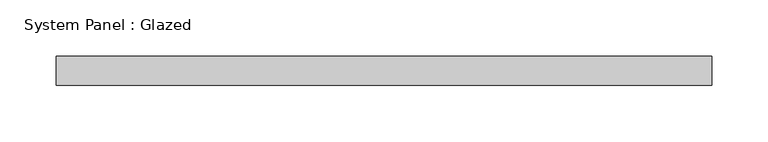
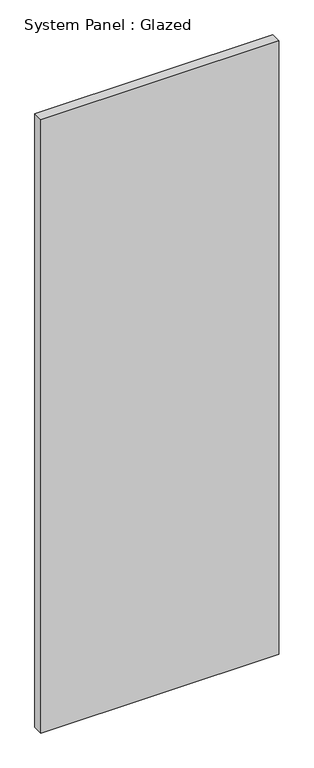
"""IFC4 building model written with IfcOpenShell, lengths in millimetres: plate geometry, System Panel : Glazed."""

from ifc_helpers import new_model, si_unit, origin, origin_with_axes, place, context, project, spatial, polyline, outline, extrude, source, transform, mapped, element, save


def system_panel_glazed_51fb9f70(model_context):
    return source(origin(), model_context, "Body", "SweptSolid", [
        extrude(outline(polyline([(289.9833333, 19.05), (-289.9833333, 19.05), (-289.9833333, 44.45), (289.9833333, 44.45), (289.9833333, 19.05)])), origin_with_axes(), (0.0, 0.0, 1.0), 1581.0857893),
    ])


if __name__ == "__main__":
    model = new_model("IFC4")
    model_context = context("Model", 3, world=origin())
    ifc_project = project(units=[si_unit("LENGTHUNIT", "METRE", prefix="MILLI")], contexts=[model_context])
    site = spatial("IfcSite", under=ifc_project)
    building = spatial("IfcBuilding", under=site)
    placement = place(None, origin())
    system_panel_glazed_shape = system_panel_glazed_51fb9f70(model_context)
    element("IfcPlate", 1, ObjectType="System Panel : Glazed", at=placement, inside=building, context=model_context, shape_type="MappedRepresentation", body=[
        mapped(system_panel_glazed_shape, transform((0.0, 0.0, 0.0), x_axis=(1.0, 0.0, 0.0), y_axis=(0.0, 1.0, 0.0), z_axis=(0.0, 0.0, 1.0))),
    ])
    save(model, "model.ifc")

# Revit data of these elements
# Type "System Panel : Glazed"
#   Construction Type Id = "GSP4R"
#   Analytic Construction = "1/8 in Pilkington single glazing"
#   Visual Light Transmittance = 0.9
#   Solar Heat Gain Coefficient = 0.86
#   Heat Transfer Coefficient (U) = 1.18115 BTU/(h·ft²·°F)
# Element 1 (IfcPlate, "System Panel : Glazed")
#   Materials on its faces: "Glass"
# Materials
#   "Glass": class "Glass", colour RGB 0 128 192, transparency 0.75, Description = "Soda Lime Glass", Cost = 0
